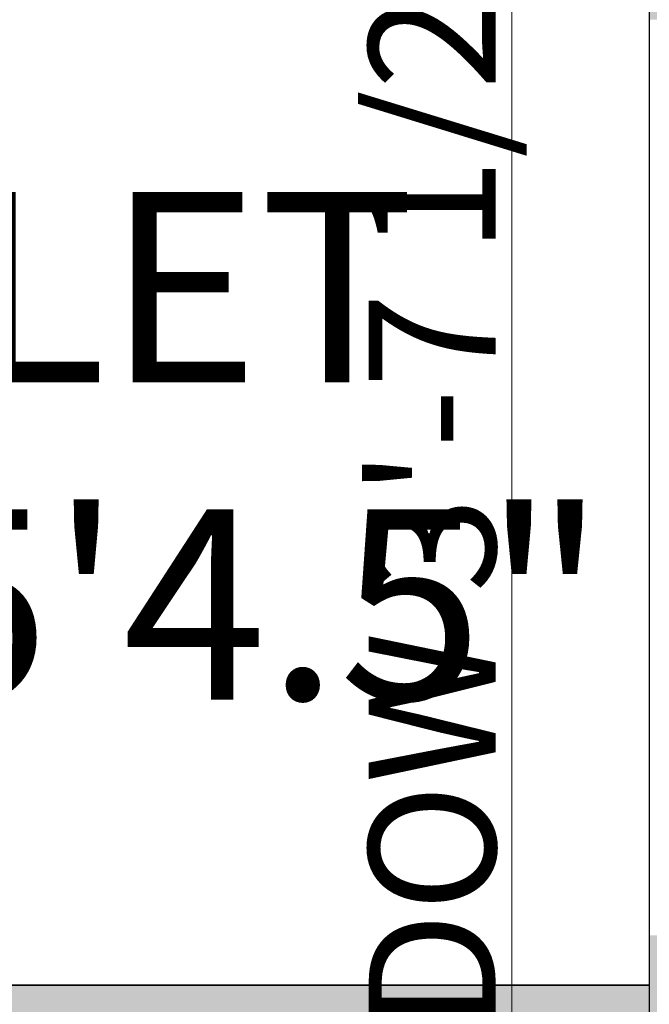
# Model space of a CAD drawing. Units: inches. Extents: x 2696 to 3240, y 1564 to 2310.
# Tile 36 of 76: x 3161 to 3191, y 1699 to 1745. Entities that reach past the tile are written whole.
import ezdxf

# ---------------------------------------------------------------- set-up
doc = ezdxf.new("R2010")
doc.units = ezdxf.units.IN
for name, color, linetype, lineweight in [('A-ANNO-DIMS', 3, 'Continuous', 18), ('A-AREA-IDEN', 7, 'Continuous', 18), ('A-WALL', 7, 'Continuous', 35), ('A-WALL-PATT', 9, 'Continuous', 13)]:
    doc.layers.add(name, color=color, linetype=linetype, lineweight=lineweight)
doc.styles.add('TIMES NEW', font='times.ttf')
doc.styles.add('YQ_DIM', font='SUPEROS.SHX', dxfattribs={"width": 0.8, "bigfont": 'HZDX.SHX'})
doc.dimstyles.new('Siddhuu', dxfattribs={"dimtxt": 6, "dimasz": 2.5, "dimexe": 1.25, "dimexo": 0.625, "dimtad": 1, "dimdec": 1, "dimlunit": 4, "dimtxsty": 'TIMES NEW', "dimcen": 2.5, "dimclrd": 256, "dimclre": 1, "dimclrt": 7, "dimadec": 0, "dimazin": 0, "dimtfac": 1, "dimtdec": 1, "dimtmove": 0, "dimatfit": 3, "dimfxl": 1, "dimtolj": 1, "dimlwd": -1, "dimarcsym": 0})

# ---------------------------------------------------------------- blocks, each defined once
blk = doc.blocks.new('*D26')
at = {"layer": 'A-ANNO-DIMS', "transparency": 16777216}
for p, q in [((3184.115, 1676.355), (3184.115, 1772.168)), ((3184.115, 1635.548), (3184.115, 1673.855))]:
    blk.add_line(p, q, dxfattribs=at)
at = {"layer": 'A-ANNO-DIMS', "color": 1, "lineweight": -2, "transparency": 16777216}
for p, q in [((3189.986, 1676.355), (3182.865, 1676.355)), ((3189.986, 1633.048), (3182.865, 1633.048))]:
    blk.add_line(p, q, dxfattribs=at)
at = {"layer": 'A-ANNO-DIMS', "transparency": 16777216}
for points in [[(3183.699, 1673.855), (3184.532, 1673.855), (3184.115, 1676.355)], [(3183.699, 1635.548), (3184.532, 1635.548), (3184.115, 1633.048)]]:
    blk.add_solid(points, dxfattribs=at)
at = {"layer": 'Defpoints', "color": 0, "transparency": 16777216}
for p in [(3184.115, 1676.355), (3190.611, 1676.355), (3190.611, 1633.048)]:
    blk.add_point(p, dxfattribs=at)
at = {"layer": 'A-ANNO-DIMS', "color": 7, "transparency": 16777216, "insert": (3180.348, 1725.511), "char_height": 6, "attachment_point": 5, "rotation": 90, "style": 'TIMES NEW'}
blk.add_mtext('\\A1;WINDOW 3\'-7 1/2" TYP.', dxfattribs=at)
blk = doc.blocks.new('*D52')
at = {"layer": 'A-ANNO-DIMS', "color": 1, "lineweight": -2, "transparency": 16777216}
for p, q in [((3148.611, 1979.576), (3148.611, 1568.951)), ((3190.611, 1979.576), (3190.611, 1568.951))]:
    blk.add_line(p, q, dxfattribs=at)
at = {"layer": 'A-ANNO-DIMS', "transparency": 16777216}
blk.add_line((3151.111, 1570.201), (3188.111, 1570.201), dxfattribs=at)
for points in [[(3151.111, 1570.618), (3151.111, 1569.784), (3148.611, 1570.201)], [(3188.111, 1570.618), (3188.111, 1569.784), (3190.611, 1570.201)]]:
    blk.add_solid(points, dxfattribs=at)
at = {"layer": 'Defpoints', "color": 0, "transparency": 16777216}
for p in [(3148.611, 1980.201), (3190.611, 1980.201), (3190.611, 1570.201)]:
    blk.add_point(p, dxfattribs=at)
at = {"layer": 'A-ANNO-DIMS', "color": 7, "transparency": 16777216, "insert": (3169.611, 1573.878), "char_height": 6, "attachment_point": 5, "style": 'TIMES NEW'}
blk.add_mtext('\\A1;3\'-6"', dxfattribs=at)
blk = doc.blocks.new('*D56')
at = {"layer": 'A-ANNO-DIMS', "color": 1, "lineweight": -2, "transparency": 16777216}
for p, q in [((2966.334, 1884.201), (3235.861, 1884.201)), ((2966.334, 1665.201), (3235.861, 1665.201))]:
    blk.add_line(p, q, dxfattribs=at)
at = {"layer": 'A-ANNO-DIMS', "transparency": 16777216}
blk.add_line((3234.611, 1667.701), (3234.611, 1881.701), dxfattribs=at)
for points in [[(3234.195, 1881.701), (3235.028, 1881.701), (3234.611, 1884.201)], [(3234.195, 1667.701), (3235.028, 1667.701), (3234.611, 1665.201)]]:
    blk.add_solid(points, dxfattribs=at)
at = {"layer": 'Defpoints', "color": 0, "transparency": 16777216}
for p in [(2965.709, 1884.201), (3234.611, 1884.201), (2965.709, 1665.201)]:
    blk.add_point(p, dxfattribs=at)
at = {"layer": 'A-ANNO-DIMS', "color": 7, "transparency": 16777216, "insert": (3230.934, 1774.701), "char_height": 6, "attachment_point": 5, "rotation": 90, "style": 'TIMES NEW'}
blk.add_mtext('\\A1;18\'-3"', dxfattribs=at)

msp = doc.modelspace()

# ---------------------------------------------------------------- hatches: boundary and pattern name
at = {"layer": 'A-WALL-PATT', "transparency": 33554556}
h = msp.add_hatch(color=256, dxfattribs=at)
h.dxf.hatch_style = 1
h.paths.add_polyline_path([(2879.111, 2253.201), (2905.91, 2253.201), (2905.91, 2262.201), (2841.889, 2262.201), (2841.889, 2253.201), (2870.111, 2253.201), (2870.111, 2176.601), (2965.709, 2176.601), (2965.709, 2206.701), (2973.583, 2206.701), (2973.583, 2215.701), (2965.709, 2215.701), (2965.709, 2262.201), (2929.91, 2262.201), (2929.91, 2253.201), (2956.709, 2253.201), (2956.709, 2185.601), (2879.111, 2185.601)])
h.paths.add_polyline_path([(2782.834, 2262.201), (2745.611, 2262.201), (2745.611, 2228.729), (2754.611, 2228.729), (2754.611, 2253.201), (2782.834, 2253.201)])
h.paths.add_polyline_path([(2754.611, 2136.201), (2965.709, 2136.201), (2965.709, 2145.201), (2879.111, 2145.201), (2879.111, 2147.074), (2877.34, 2147.074), (2870.111, 2147.074), (2870.111, 2145.201), (2754.611, 2145.201), (2754.611, 2169.674), (2745.611, 2169.674), (2745.611, 2000.201), (2754.611, 2000.201), (2754.611, 2019.201), (2849.083, 2019.201), (2849.083, 2023.701), (2841.209, 2023.701), (2841.209, 2051.827), (2836.709, 2051.827), (2836.709, 2023.701), (2754.611, 2023.701), (2754.611, 2091.201), (2836.709, 2091.201), (2836.709, 2087.827), (2841.209, 2087.827), (2841.209, 2095.701), (2754.611, 2095.701)])
h.paths.add_polyline_path([(2965.709, 2136.201), (2956.709, 2136.201), (2956.709, 2023.701), (2885.083, 2023.701), (2885.083, 2019.201), (2956.709, 2019.201), (2956.709, 1950.575), (2965.709, 1950.575), (2965.709, 1980.201), (2973.583, 1980.201), (2973.583, 1989.201), (2965.709, 1989.201)])
h.paths.add_polyline_path([(2754.611, 1906.701), (2880.209, 1906.701), (2884.709, 1906.701), (2956.709, 1906.701), (2956.709, 1792.701), (2944.709, 1792.701), (2944.709, 1783.701), (2956.709, 1783.701), (2956.709, 1740.201), (2884.709, 1740.201), (2884.709, 1783.701), (2896.709, 1783.701), (2896.709, 1792.701), (2884.709, 1792.701), (2884.709, 1846.701), (2880.209, 1846.701), (2880.209, 1740.201), (2754.611, 1740.201), (2754.611, 1777.201), (2745.611, 1777.201), (2745.611, 1692.701), (2754.611, 1692.701), (2754.611, 1731.201), (2956.709, 1731.201), (2956.709, 1723.327), (2965.709, 1723.327), (2965.709, 1884.201), (2973.583, 1884.201), (2973.583, 1893.201), (2965.709, 1893.201), (2965.709, 1914.575), (2956.709, 1914.575), (2956.709, 1911.201), (2754.611, 1911.201), (2754.611, 1930.201), (2745.611, 1930.201), (2745.611, 1817.201), (2754.611, 1817.201), (2754.611, 1854.201), (2826.611, 1854.201), (2826.611, 1868.827), (2822.111, 1868.827), (2822.111, 1858.701), (2754.611, 1858.701)])
h.paths.add_polyline_path([(2965.709, 1656.201), (3008.237, 1656.201), (3008.237, 1665.201), (2965.709, 1665.201), (2965.709, 1693.327), (2956.709, 1693.327), (2956.709, 1686.201), (2934.583, 1686.201), (2934.583, 1681.701), (2956.709, 1681.701), (2956.709, 1614.201), (2896.709, 1614.201), (2896.709, 1681.701), (2904.583, 1681.701), (2904.583, 1686.201), (2892.209, 1686.201), (2892.209, 1614.201), (2858.41, 1614.201), (2858.41, 1605.201), (2965.709, 1605.201)])
h.paths.add_polyline_path([(2788.41, 1614.201), (2754.611, 1614.201), (2754.611, 1652.701), (2745.611, 1652.701), (2745.611, 1605.201), (2788.41, 1605.201)])
h.paths.add_polyline_path([(3199.611, 1633.048), (3190.611, 1633.048), (3190.611, 1614.201), (3082.611, 1614.201), (3082.611, 1665.201), (3070.237, 1665.201), (3070.237, 1656.201), (3078.111, 1656.201), (3078.111, 1605.201), (3199.611, 1605.201)])
h.paths.add_polyline_path([(3199.611, 1702.048), (3190.611, 1702.048), (3190.611, 1699.701), (3106.611, 1699.701), (3106.611, 1747.701), (3190.611, 1747.701), (3190.611, 1752.201), (3082.611, 1752.201), (3082.611, 1760.075), (3078.111, 1760.075), (3078.111, 1747.701), (3102.111, 1747.701), (3102.111, 1699.701), (3078.111, 1699.701), (3078.111, 1695.201), (3190.611, 1695.201), (3190.611, 1676.355), (3199.611, 1676.355)])
h.paths.add_polyline_path([(3199.611, 1783.201), (3190.611, 1783.201), (3190.611, 1745.355), (3199.611, 1745.355)])
h.paths.add_polyline_path([(3082.611, 1884.201), (3190.611, 1884.201), (3190.611, 1853.201), (3199.611, 1853.201), (3199.611, 1901.701), (3190.611, 1901.701), (3190.611, 1893.201), (3005.583, 1893.201), (3005.583, 1891.281), (3005.583, 1884.201), (3078.111, 1884.201), (3078.111, 1792.075), (3082.611, 1792.075)])
h.paths.add_polyline_path([(3199.611, 1994.701), (3190.611, 1994.701), (3190.611, 1989.201), (3073.709, 1989.201), (3073.709, 2034.201), (3069.209, 2034.201), (3069.209, 1989.201), (3005.583, 1989.201), (3005.583, 1980.201), (3190.611, 1980.201), (3190.611, 1971.701), (3199.611, 1971.701)])
h.paths.add_polyline_path([(3199.611, 2155.201), (3190.611, 2155.201), (3190.611, 2064.701), (3199.611, 2064.701)])
h.paths.add_polyline_path([(3190.611, 2074.701), (3106.611, 2074.701), (3106.611, 2122.701), (3190.611, 2122.701), (3190.611, 2127.201), (3082.709, 2127.201), (3082.709, 2135.075), (3073.709, 2135.075), (3073.709, 2122.701), (3102.111, 2122.701), (3102.111, 2074.701), (3069.209, 2074.701), (3069.209, 2070.201), (3190.611, 2070.201)])
h.paths.add_polyline_path([(3082.709, 2253.201), (3190.611, 2253.201), (3190.611, 2225.201), (3199.611, 2225.201), (3199.611, 2262.201), (3073.709, 2262.201), (3073.709, 2215.701), (3035.583, 2215.701), (3035.583, 2206.701), (3073.709, 2206.701), (3073.709, 2171.075), (3082.709, 2171.075)])

# ---------------------------------------------------------------- linework, layer by layer
at = {"layer": 'A-WALL'}
msp.add_line((3106.611, 1699.701), (3190.611, 1699.701), dxfattribs=at)

# ---------------------------------------------------------------- texts
at = {"layer": 'A-AREA-IDEN', "insert": (3138.221, 1737.206), "char_height": 9, "attachment_point": 1, "style": 'YQ_DIM'}
msp.add_mtext_dynamic_manual_height_columns('TOILET\\P5\'X5\'4.5"', width=48.00324, gutter_width=12.5, heights=[0], dxfattribs=at)

# ---------------------------------------------------------------- dimensions: what is measured, and where the dimension line sits
at = {"layer": 'A-ANNO-DIMS'}
dim = msp.add_linear_dim(base=(3190.611, 1570.201), p1=(3148.611, 1980.201), p2=(3190.611, 1980.201), dimstyle='Siddhuu', override={"dimdec": 1, "dimlfac": 1, "dimrnd": 0, "dimzin": 1, "dimdsep": 46, "dimlunit": 4, "dimfrac": 2}, dxfattribs=at)
dim.commit()
dim.dimension.update_dxf_attribs({"geometry": '*D52', "text_midpoint": (3169.611, 1573.878)})
dim = msp.add_linear_dim(base=(3234.611, 1884.201), p1=(2965.709, 1665.201), p2=(2965.709, 1884.201), angle=90, dimstyle='Siddhuu', override={"dimdec": 1, "dimlfac": 1, "dimrnd": 0, "dimzin": 1, "dimdsep": 46, "dimlunit": 4, "dimfrac": 2}, dxfattribs=at)
dim.commit()
dim.dimension.update_dxf_attribs({"geometry": '*D56', "text_midpoint": (3230.934, 1774.701)})
dim = msp.add_linear_dim(base=(3184.115, 1676.355), p1=(3190.611, 1633.048), p2=(3190.611, 1676.355), angle=90, text='WINDOW <> TYP.', dimstyle='Siddhuu', override={"dimdec": 1, "dimlfac": 1, "dimrnd": 0, "dimzin": 1, "dimdsep": 46, "dimlunit": 4, "dimfrac": 2}, dxfattribs=at)
dim.commit()
dim.dimension.update_dxf_attribs({"geometry": '*D26', "text_midpoint": (3180.348, 1725.511)})

doc.saveas('drawing.dxf')
